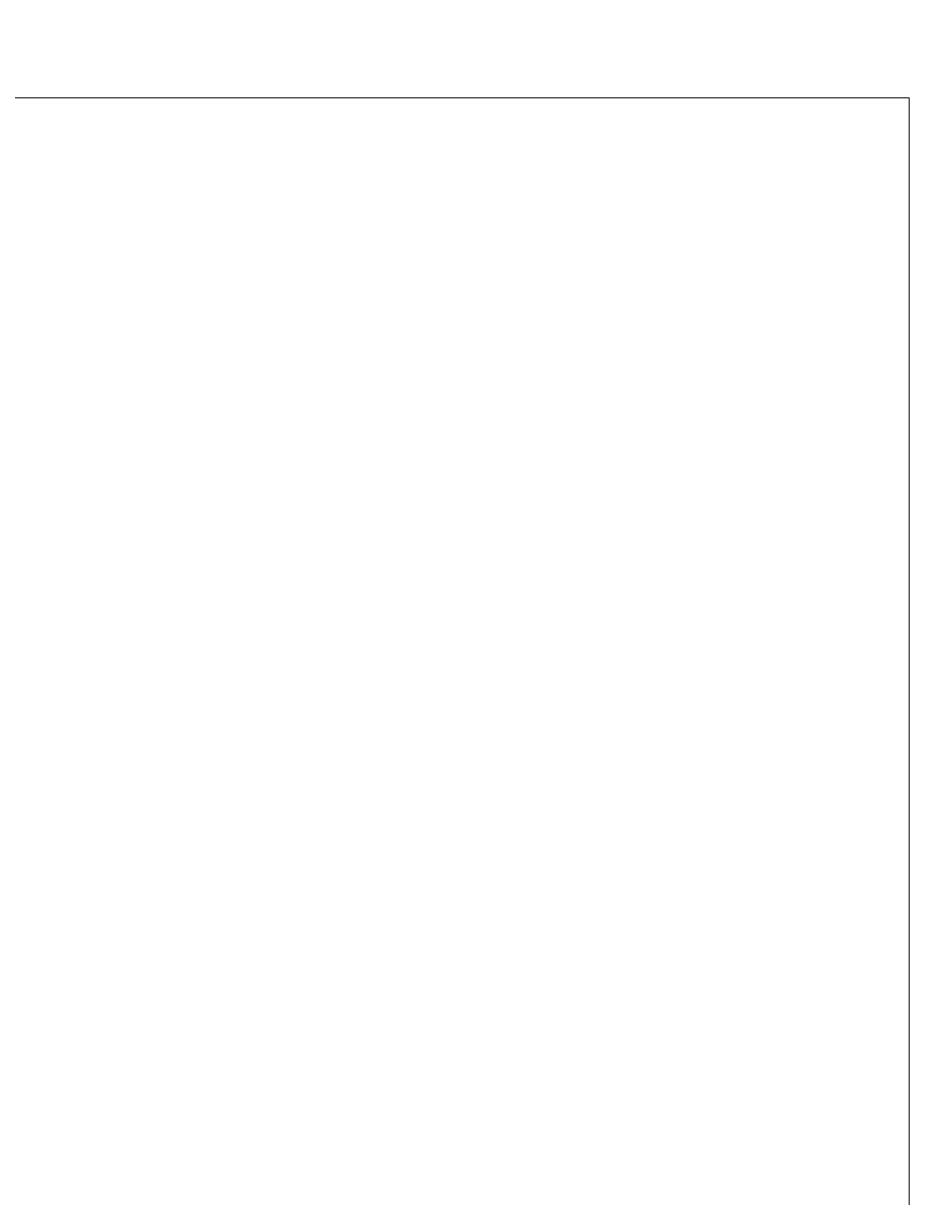
# Model space of a CAD drawing. Units: inches. Extents: x -301 to 715, y -607 to 364.
# Tile 73 of 141: x -164 to -123, y -26 to 26. Entities that reach past the tile are written whole.
import ezdxf

# ---------------------------------------------------------------- set-up
doc = ezdxf.new("R2010")
doc.units = ezdxf.units.IN
doc.header["$MEASUREMENT"] = 0
doc.layers.add('A-ANNO-DIMS', color=2, linetype='Continuous', lineweight=18)
doc.layers.add('A-FURN', color=8, linetype='Continuous', lineweight=18)
doc.styles.get("Standard").update_dxf_attribs({"font": 'arial.ttf'})
doc.dimstyles.get("Standard").update_dxf_attribs({"dimtxt": 0.18, "dimasz": 0.18, "dimexe": 0.18, "dimexo": 0.0625, "dimgap": 0.09, "dimtad": 0, "dimtih": 1, "dimtoh": 1, "dimdec": 1, "dimzin": 0, "dimdsep": 46, "dimlunit": 4, "dimtxsty": 'Standard', "dimcen": 0.09, "dimclrd": 3, "dimclre": 4, "dimclrt": 6, "dimadec": 0, "dimazin": 0, "dimtfac": 1, "dimtdec": 1, "dimtofl": 0, "dimtmove": 0, "dimatfit": 3, "dimfxl": 1, "dimtfill": 2, "dimtfillclr": 51, "dimtolj": 1, "dimtzin": 0, "dimarcsym": 0})

# ---------------------------------------------------------------- blocks, each defined once
blk = doc.blocks.new('Bed - Queen')
for p, q in [((59.99999, 0), (59.99999, -80.00003)), ((59.99999, -80.00003), (0, -80.00003))]:
    blk.add_line(p, q)
blk = doc.blocks.new('*D151')
at = {"layer": 'A-ANNO-DIMS', "color": 4, "lineweight": -2, "transparency": 16777216}
for p, q in [((-204.603, -223.755), (-204.603, 359.612)), ((-45.603, -214.755), (-45.603, 359.612))]:
    blk.add_line(p, q, dxfattribs=at)
at = {"layer": 'A-ANNO-DIMS', "color": 3, "lineweight": -2, "transparency": 16777216}
for p, q in [((-204.423, 359.432), (-125.494, 359.432)), ((-45.783, 359.432), (-124.713, 359.432))]:
    blk.add_line(p, q, dxfattribs=at)
at = {"layer": 'A-ANNO-DIMS', "color": 3, "transparency": 16777216}
for points in [[(-204.423, 359.462), (-204.423, 359.402), (-204.603, 359.432)], [(-45.783, 359.462), (-45.783, 359.402), (-45.603, 359.432)]]:
    blk.add_solid(points, dxfattribs=at)
at = {"layer": 'Defpoints', "color": 0, "transparency": 16777216}
for p in [(-45.603, 359.432), (-45.603, -214.818), (-204.603, -223.818)]:
    blk.add_point(p, dxfattribs=at)
at = {"layer": 'A-ANNO-DIMS', "color": 6, "transparency": 16777216, "insert": (-125.103, 359.432), "char_height": 0.18, "attachment_point": 5, "bg_fill": 1, "box_fill_scale": 1.25, "bg_fill_color": 51, "bg_fill_transparency": 0}
blk.add_mtext('\\A1;13\'-3"', dxfattribs=at)

msp = doc.modelspace()

# ---------------------------------------------------------------- block references
at = {"layer": 'A-FURN', "xscale": 0.8856750462000775, "yscale": 0.8856750462000775, "zscale": 0.8856750462000775, "rotation": 90}
msp.add_blockref('Bed - Queen', (-195.207, -30.095), dxfattribs=at)

# ---------------------------------------------------------------- dimensions: what is measured, and where the dimension line sits
at = {"layer": 'A-ANNO-DIMS'}
dim = msp.add_linear_dim(base=(-45.603, 359.432), p1=(-204.603, -223.818), p2=(-45.603, -214.818), dimstyle='Standard', override={"dimdec": 1, "dimlfac": 1, "dimrnd": 0, "dimzin": 1, "dimdsep": 46, "dimlunit": 4, "dimfrac": 2}, dxfattribs=at)
dim.commit()
dim.dimension.update_dxf_attribs({"geometry": '*D151', "text_midpoint": (-125.103, 359.432)})

doc.saveas('drawing.dxf')
